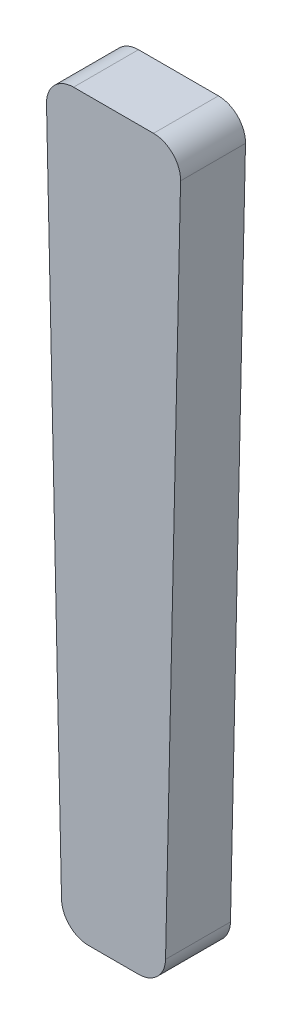
from build123d import *

# Parameters (mm, degrees)
COTTER_BODY_DEPTH = 6


with BuildPart() as part:
    # Cotter Profile Sketch → Cotter Body (new, symmetric)
    with BuildSketch(Plane.XY):
        with BuildLine():
            Line((-7.388671752, 77.068898934), (7.388671752, 77.068898934))
            ThreePointArc((7.388671752, 77.068898934), (10.962916131, 75.565293809), (12.387459643, 71.958809784))
            Line((12.387459643, 71.958809784), (9.612540357, -54.041190216))
            ThreePointArc((9.612540357, -54.041190216), (8.110147341, -57.505345445), (4.613752466, -58.931101066))
            Line((4.613752466, -58.931101066), (-4.613752466, -58.931101066))
            ThreePointArc((-4.613752466, -58.931101066), (-8.110147341, -57.505345445), (-9.612540357, -54.041190216))
            Line((-9.612540357, -54.041190216), (-12.387459643, 71.958809784))
            ThreePointArc((-12.387459643, 71.958809784), (-10.962916131, 75.565293809), (-7.388671752, 77.068898934))
        make_face()
    extrude(amount=COTTER_BODY_DEPTH, both=True)


solid = part.part
